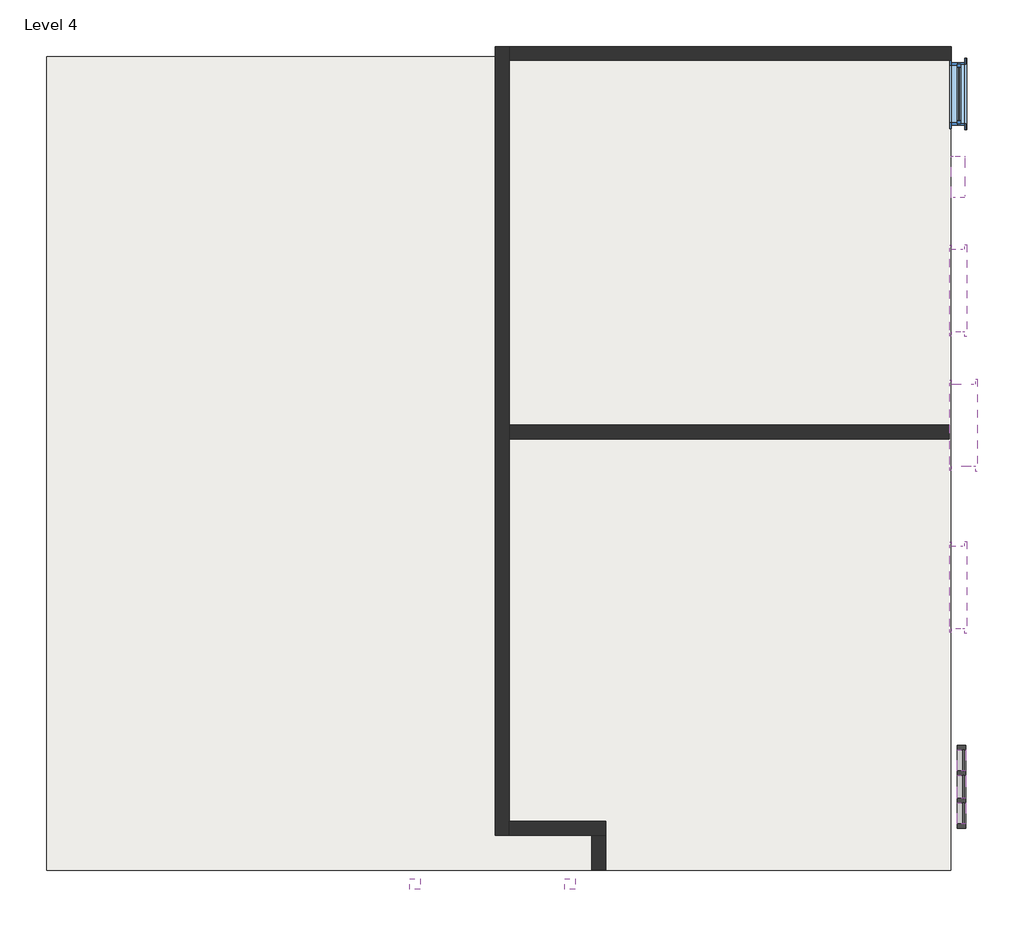
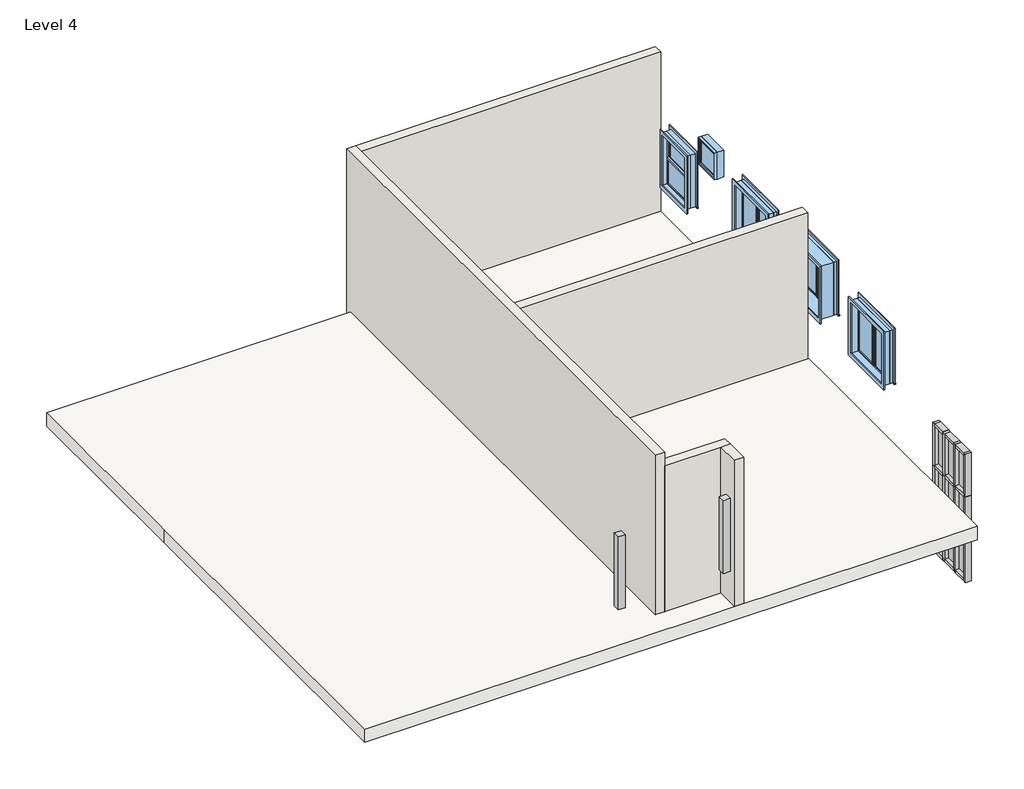
# One storey: 24 members, 9 plates, 5 walls, 5 windows, 2 proxies, 1 roof.
"""IFC4 building model written with IfcOpenShell, lengths in millimetres."""

from ifc_helpers import new_model, si_unit, frame, origin, place, context, project, spatial, polyline, outline, extrude, faceted_brep, transform, mapped, element, save
from components import member_ff1b7d8f, member_5ad95953, member_5aeb4b7d, member_9850ab14, member_fc2bd130, member_09852e99, system_panel_glazed_48942baa, system_panel_glazed_b83167b9, system_panel_glazed_fcfd29d5, system_panel_glazed_c81023b1, window_0862ab64, window_6544a982, window_31198920, window_6846e476

model = new_model("IFC4")

# Units and contexts
model_context = context("Model", 3, world=origin())
ifc_project = project(units=[si_unit("LENGTHUNIT", "METRE", prefix="MILLI")], contexts=[model_context])

# Site, building, storey
site = spatial("IfcSite", under=ifc_project)
building = spatial("IfcBuilding", under=site)
storey = spatial("IfcBuildingStorey", under=building, Name="Level 4", Elevation=10972.8)

# Proxies
placement = place(None, origin())
element("IfcBuildingElementProxy", 1, Name="Cornice", ObjectType="Cornice", at=placement, inside=storey, context=model_context, shape_type="SweptSolid", body=[
    extrude(outline(polyline([(-6354.4547188, -909.5189974), (-6354.4547188, -1061.9189974), (-6506.8547188, -1061.9189974), (-6506.8547188, -909.5189974), (-6354.4547188, -909.5189974)])), frame((0.0, 0.0, 12313.3022407), z_axis=(0.0, 0.0, 1.0), x_axis=(1.0, 0.0, 0.0)), (0.0, 0.0, 1.0), 1676.4),
])
element("IfcBuildingElementProxy", 2, Name="Cornice", ObjectType="Cornice", at=placement, inside=storey, context=model_context, shape_type="SweptSolid", body=[
    extrude(outline(polyline([(-4073.2084212, -909.5189974), (-4073.2084212, -1061.9189974), (-4225.6084212, -1061.9189974), (-4225.6084212, -909.5189974), (-4073.2084212, -909.5189974)])), frame((0.0, 0.0, 12347.4321664), z_axis=(0.0, 0.0, 1.0), x_axis=(1.0, 0.0, 0.0)), (0.0, 0.0, 1.0), 1676.4),
])

# Members
member_shape = member_ff1b7d8f(model_context)
element("IfcMember", 3, ObjectType="Rectangular Mullion : 2.5\" x 5\" rectangular", at=placement, inside=storey, context=model_context, shape_type="MappedRepresentation", body=[
    mapped(member_shape, transform((1611.5254876, 617.0832725, 9576.1019988), x_axis=(0.0, 0.0, -1.0), y_axis=(-1.0, 0.0, 0.0), z_axis=(0.0, 1.0, 0.0))),
])
member_2_shape = member_5ad95953(model_context)
element("IfcMember", 4, ObjectType="Rectangular Mullion : 2.5\" x 5\" rectangular", at=placement, inside=storey, context=model_context, shape_type="MappedRepresentation", body=[
    mapped(member_2_shape, transform((1611.5254876, 210.6832725, 9576.1019988), x_axis=(0.0, 0.0, -1.0), y_axis=(-1.0, 0.0, 0.0), z_axis=(0.0, 1.0, 0.0))),
])
element("IfcMember", 5, ObjectType="Rectangular Mullion : 2.5\" x 5\" rectangular", at=placement, inside=storey, context=model_context, shape_type="MappedRepresentation", body=[
    mapped(member_2_shape, transform((1611.5254876, 991.7332725, 9576.1019988), x_axis=(0.0, 0.0, -1.0), y_axis=(-1.0, 0.0, 0.0), z_axis=(0.0, 1.0, 0.0))),
])
member_3_shape = member_5aeb4b7d(model_context)
element("IfcMember", 6, ObjectType="Rectangular Mullion : 2.5\" x 5\" rectangular", at=placement, inside=storey, context=model_context, shape_type="MappedRepresentation", body=[
    mapped(member_3_shape, transform((1611.5254876, 274.1832725, 10558.2353321), x_axis=(0.0, 0.0, 1.0), y_axis=(-1.0, 0.0, 0.0), z_axis=(0.0, -1.0, 0.0))),
])
element("IfcMember", 7, ObjectType="Rectangular Mullion : 2.5\" x 5\" rectangular", at=placement, inside=storey, context=model_context, shape_type="MappedRepresentation", body=[
    mapped(member_3_shape, transform((1611.5254876, 274.1832725, 11540.3686655), x_axis=(0.0, 0.0, 1.0), y_axis=(-1.0, 0.0, 0.0), z_axis=(0.0, -1.0, 0.0))),
])
member_4_shape = member_9850ab14(model_context)
element("IfcMember", 8, ObjectType="Rectangular Mullion : 2.5\" x 5\" rectangular", at=placement, inside=storey, context=model_context, shape_type="MappedRepresentation", body=[
    mapped(member_4_shape, transform((1611.5254876, -100.4667275, 10558.2353321), x_axis=(0.0, 0.0, 1.0), y_axis=(-1.0, 0.0, 0.0), z_axis=(0.0, -1.0, 0.0))),
])
element("IfcMember", 9, ObjectType="Rectangular Mullion : 2.5\" x 5\" rectangular", at=placement, inside=storey, context=model_context, shape_type="MappedRepresentation", body=[
    mapped(member_4_shape, transform((1611.5254876, 680.5832725, 10558.2353321), x_axis=(0.0, 0.0, 1.0), y_axis=(-1.0, 0.0, 0.0), z_axis=(0.0, -1.0, 0.0))),
])
element("IfcMember", 10, ObjectType="Rectangular Mullion : 2.5\" x 5\" rectangular", at=placement, inside=storey, context=model_context, shape_type="MappedRepresentation", body=[
    mapped(member_4_shape, transform((1611.5254876, -100.4667275, 11540.3686655), x_axis=(0.0, 0.0, 1.0), y_axis=(-1.0, 0.0, 0.0), z_axis=(0.0, -1.0, 0.0))),
])
element("IfcMember", 11, ObjectType="Rectangular Mullion : 2.5\" x 5\" rectangular", at=placement, inside=storey, context=model_context, shape_type="MappedRepresentation", body=[
    mapped(member_4_shape, transform((1611.5254876, 680.5832725, 11540.3686655), x_axis=(0.0, 0.0, 1.0), y_axis=(-1.0, 0.0, 0.0), z_axis=(0.0, -1.0, 0.0))),
])
element("IfcMember", 12, ObjectType="Rectangular Mullion : 2.5\" x 5\" rectangular", at=placement, inside=storey, context=model_context, shape_type="MappedRepresentation", body=[
    mapped(member_2_shape, transform((1611.5254876, 680.5832725, 12522.5019988), x_axis=(0.0, 0.0, 1.0), y_axis=(-1.0, 0.0, 0.0), z_axis=(0.0, -1.0, 0.0))),
])
element("IfcMember", 13, ObjectType="Rectangular Mullion : 2.5\" x 5\" rectangular", at=placement, inside=storey, context=model_context, shape_type="MappedRepresentation", body=[
    mapped(member_2_shape, transform((1611.5254876, -100.4667275, 12522.5019988), x_axis=(0.0, 0.0, 1.0), y_axis=(-1.0, 0.0, 0.0), z_axis=(0.0, -1.0, 0.0))),
])
element("IfcMember", 14, ObjectType="Rectangular Mullion : 2.5\" x 5\" rectangular", at=placement, inside=storey, context=model_context, shape_type="MappedRepresentation", body=[
    mapped(member_shape, transform((1611.5254876, 274.1832725, 12522.5019988), x_axis=(0.0, 0.0, 1.0), y_axis=(-1.0, 0.0, 0.0), z_axis=(0.0, -1.0, 0.0))),
])
member_5_shape = member_fc2bd130(model_context)
element("IfcMember", 15, ObjectType="Rectangular Mullion : 2.5\" x 5\" rectangular", at=placement, inside=storey, context=model_context, shape_type="MappedRepresentation", body=[
    mapped(member_5_shape, transform((1611.5254876, 242.4332725, 9576.1019988), x_axis=(0.0, -1.0, 0.0), y_axis=(-1.0, 0.0, 0.0), z_axis=(0.0, 0.0, -1.0))),
])
element("IfcMember", 16, ObjectType="Rectangular Mullion : 2.5\" x 5\" rectangular", at=placement, inside=storey, context=model_context, shape_type="MappedRepresentation", body=[
    mapped(member_5_shape, transform((1611.5254876, 648.8332725, 9576.1019988), x_axis=(0.0, -1.0, 0.0), y_axis=(-1.0, 0.0, 0.0), z_axis=(0.0, 0.0, -1.0))),
])
element("IfcMember", 17, ObjectType="Rectangular Mullion : 2.5\" x 5\" rectangular", at=placement, inside=storey, context=model_context, shape_type="MappedRepresentation", body=[
    mapped(member_5_shape, transform((1611.5254876, 242.4332725, 10558.2353321), x_axis=(0.0, -1.0, 0.0), y_axis=(-1.0, 0.0, 0.0), z_axis=(0.0, 0.0, -1.0))),
])
element("IfcMember", 18, ObjectType="Rectangular Mullion : 2.5\" x 5\" rectangular", at=placement, inside=storey, context=model_context, shape_type="MappedRepresentation", body=[
    mapped(member_5_shape, transform((1611.5254876, 648.8332725, 10558.2353321), x_axis=(0.0, -1.0, 0.0), y_axis=(-1.0, 0.0, 0.0), z_axis=(0.0, 0.0, -1.0))),
])
element("IfcMember", 19, ObjectType="Rectangular Mullion : 2.5\" x 5\" rectangular", at=placement, inside=storey, context=model_context, shape_type="MappedRepresentation", body=[
    mapped(member_5_shape, transform((1611.5254876, 242.4332725, 11540.3686655), x_axis=(0.0, -1.0, 0.0), y_axis=(-1.0, 0.0, 0.0), z_axis=(0.0, 0.0, -1.0))),
])
element("IfcMember", 20, ObjectType="Rectangular Mullion : 2.5\" x 5\" rectangular", at=placement, inside=storey, context=model_context, shape_type="MappedRepresentation", body=[
    mapped(member_5_shape, transform((1611.5254876, 648.8332725, 11540.3686655), x_axis=(0.0, -1.0, 0.0), y_axis=(-1.0, 0.0, 0.0), z_axis=(0.0, 0.0, -1.0))),
])
member_6_shape = member_09852e99(model_context)
element("IfcMember", 21, ObjectType="Rectangular Mullion : 2.5\" x 5\" rectangular", at=placement, inside=storey, context=model_context, shape_type="MappedRepresentation", body=[
    mapped(member_6_shape, transform((1611.5254876, 1055.2332725, 11540.3686655), x_axis=(0.0, 1.0, 0.0), y_axis=(-1.0, 0.0, 0.0), z_axis=(0.0, 0.0, 1.0))),
])
element("IfcMember", 22, ObjectType="Rectangular Mullion : 2.5\" x 5\" rectangular", at=placement, inside=storey, context=model_context, shape_type="MappedRepresentation", body=[
    mapped(member_6_shape, transform((1611.5254876, 1055.2332725, 10558.2353321), x_axis=(0.0, 1.0, 0.0), y_axis=(-1.0, 0.0, 0.0), z_axis=(0.0, 0.0, 1.0))),
])
element("IfcMember", 23, ObjectType="Rectangular Mullion : 2.5\" x 5\" rectangular", at=placement, inside=storey, context=model_context, shape_type="MappedRepresentation", body=[
    mapped(member_6_shape, transform((1611.5254876, 1055.2332725, 12522.5019988), x_axis=(0.0, 1.0, 0.0), y_axis=(-1.0, 0.0, 0.0), z_axis=(0.0, 0.0, 1.0))),
])
element("IfcMember", 24, ObjectType="Rectangular Mullion : 2.5\" x 5\" rectangular", at=placement, inside=storey, context=model_context, shape_type="MappedRepresentation", body=[
    mapped(member_6_shape, transform((1611.5254876, -163.9667275, 11540.3686655), x_axis=(0.0, -1.0, 0.0), y_axis=(-1.0, 0.0, 0.0), z_axis=(0.0, 0.0, -1.0))),
])
element("IfcMember", 25, ObjectType="Rectangular Mullion : 2.5\" x 5\" rectangular", at=placement, inside=storey, context=model_context, shape_type="MappedRepresentation", body=[
    mapped(member_6_shape, transform((1611.5254876, -163.9667275, 10558.2353321), x_axis=(0.0, -1.0, 0.0), y_axis=(-1.0, 0.0, 0.0), z_axis=(0.0, 0.0, -1.0))),
])
element("IfcMember", 26, ObjectType="Rectangular Mullion : 2.5\" x 5\" rectangular", at=placement, inside=storey, context=model_context, shape_type="MappedRepresentation", body=[
    mapped(member_6_shape, transform((1611.5254876, -163.9667275, 9576.1019988), x_axis=(0.0, -1.0, 0.0), y_axis=(-1.0, 0.0, 0.0), z_axis=(0.0, 0.0, -1.0))),
])

# Plates
system_panel_glazed_shape = system_panel_glazed_48942baa(model_context)
element("IfcPlate", 27, ObjectType="System Panel : Glazed", at=placement, inside=storey, context=model_context, shape_type="MappedRepresentation", body=[
    mapped(system_panel_glazed_shape, transform((1611.5254876, 445.6332725, 9639.6019988), x_axis=(0.0, -1.0, 0.0), y_axis=(1.0, 0.0, 0.0), z_axis=(0.0, 0.0, 1.0))),
])
element("IfcPlate", 28, ObjectType="System Panel : Glazed", at=placement, inside=storey, context=model_context, shape_type="MappedRepresentation", body=[
    mapped(system_panel_glazed_shape, transform((1611.5254876, 445.6332725, 11572.1186655), x_axis=(0.0, -1.0, 0.0), y_axis=(1.0, 0.0, 0.0), z_axis=(0.0, 0.0, 1.0))),
])
system_panel_glazed_2_shape = system_panel_glazed_b83167b9(model_context)
element("IfcPlate", 29, ObjectType="System Panel : Glazed", at=placement, inside=storey, context=model_context, shape_type="MappedRepresentation", body=[
    mapped(system_panel_glazed_2_shape, transform((1611.5254876, 445.6332725, 10589.9853321), x_axis=(0.0, -1.0, 0.0), y_axis=(1.0, 0.0, 0.0), z_axis=(0.0, 0.0, 1.0))),
])
system_panel_glazed_3_shape = system_panel_glazed_fcfd29d5(model_context)
element("IfcPlate", 30, ObjectType="System Panel : Glazed", at=placement, inside=storey, context=model_context, shape_type="MappedRepresentation", body=[
    mapped(system_panel_glazed_3_shape, transform((1611.5254876, 836.1582725, 9639.6019988), x_axis=(0.0, -1.0, 0.0), y_axis=(1.0, 0.0, 0.0), z_axis=(0.0, 0.0, 1.0))),
])
element("IfcPlate", 31, ObjectType="System Panel : Glazed", at=placement, inside=storey, context=model_context, shape_type="MappedRepresentation", body=[
    mapped(system_panel_glazed_3_shape, transform((1611.5254876, 55.1082725, 9639.6019988), x_axis=(0.0, -1.0, 0.0), y_axis=(1.0, 0.0, 0.0), z_axis=(0.0, 0.0, 1.0))),
])
element("IfcPlate", 32, ObjectType="System Panel : Glazed", at=placement, inside=storey, context=model_context, shape_type="MappedRepresentation", body=[
    mapped(system_panel_glazed_3_shape, transform((1611.5254876, 836.1582725, 11572.1186655), x_axis=(0.0, -1.0, 0.0), y_axis=(1.0, 0.0, 0.0), z_axis=(0.0, 0.0, 1.0))),
])
element("IfcPlate", 33, ObjectType="System Panel : Glazed", at=placement, inside=storey, context=model_context, shape_type="MappedRepresentation", body=[
    mapped(system_panel_glazed_3_shape, transform((1611.5254876, 55.1082725, 11572.1186655), x_axis=(0.0, -1.0, 0.0), y_axis=(1.0, 0.0, 0.0), z_axis=(0.0, 0.0, 1.0))),
])
system_panel_glazed_4_shape = system_panel_glazed_c81023b1(model_context)
element("IfcPlate", 34, ObjectType="System Panel : Glazed", at=placement, inside=storey, context=model_context, shape_type="MappedRepresentation", body=[
    mapped(system_panel_glazed_4_shape, transform((1611.5254876, 836.1582725, 10589.9853321), x_axis=(0.0, -1.0, 0.0), y_axis=(1.0, 0.0, 0.0), z_axis=(0.0, 0.0, 1.0))),
])
element("IfcPlate", 35, ObjectType="System Panel : Glazed", at=placement, inside=storey, context=model_context, shape_type="MappedRepresentation", body=[
    mapped(system_panel_glazed_4_shape, transform((1611.5254876, 55.1082725, 10589.9853321), x_axis=(0.0, -1.0, 0.0), y_axis=(1.0, 0.0, 0.0), z_axis=(0.0, 0.0, 1.0))),
])

# Roof
element("IfcRoof", 36, ObjectType="Generic - 12\"", at=placement, inside=storey, context=model_context, shape_type="SweptSolid", body=[
    extrude(outline(polyline([(-11850.4745124, 11192.9609482), (1452.7754876, 11192.9609482), (1452.7754876, -783.1390518), (-11850.4745124, -783.1390518), (-11850.4745124, 6786.0609482), (-11850.4745124, 11192.9609482)])), frame((0.0, 0.0, 10972.8), z_axis=(0.0, 0.0, 1.0), x_axis=(1.0, 0.0, 0.0)), (0.0, 0.0, 1.0), 304.8),
])

# Walls
element("IfcWall", 37, ObjectType="Generic - 8\"", at=placement, inside=storey, context=model_context, shape_type="Brep", body=[
    faceted_brep([(-5246.4745124, 11345.3609482, 10972.8), (-5246.4745124, -265.5667275, 10972.8), (-5246.4745124, -265.5667275, 14935.2), (-5246.4745124, 11345.3609482, 14935.2), (-5043.2745124, 11345.3609482, 10972.8), (-5043.2745124, 11345.3609482, 14935.2), (-5043.2745124, 11142.1609482, 14935.2), (-5043.2745124, -265.5667275, 14935.2), (-5043.2745124, -265.5667275, 14630.4), (-5043.2745124, -265.5667275, 10972.8), (-5043.2745124, -62.3667275, 10972.8), (-5043.2745124, 5566.8609482, 10972.8), (-5043.2745124, 5770.0609482, 10972.8), (-5043.2745124, 11142.1609482, 10972.8)], [[[0, 1, 2, 3]], [[4, 5, 6, 7, 8, 9, 10, 11, 12, 13]], [[1, 0, 4, 13, 12, 11, 10, 9]], [[3, 2, 7, 6, 5]], [[0, 3, 5, 4]], [[2, 1, 9, 8, 7]]]),
])
element("IfcWall", 38, ObjectType="Generic - 8\"", at=placement, inside=storey, context=model_context, shape_type="Brep", body=[
    faceted_brep([(-5043.2745124, 11142.1609482, 10972.8), (1459.1254876, 11142.1609482, 10972.8), (1459.1254876, 11142.1609482, 14935.2), (-5043.2745124, 11142.1609482, 14935.2), (-5043.2745124, 11345.3609482, 10972.8), (-5043.2745124, 11345.3609482, 14935.2), (1459.1254876, 11345.3609482, 14935.2), (1459.1254876, 11345.3609482, 11277.6), (1459.1254876, 11345.3609482, 10972.8)], [[[0, 1, 2, 3]], [[4, 5, 6, 7, 8]], [[1, 0, 4, 8]], [[3, 2, 6, 5]], [[1, 8, 7, 6, 2]], [[0, 3, 5, 4]]]),
])
element("IfcWall", 39, ObjectType="Generic - 8\"", at=placement, inside=storey, context=model_context, shape_type="SweptSolid", body=[
    extrude(outline(polyline([(1433.7254876, 5566.8609482), (-5043.2745124, 5566.8609482), (-5043.2745124, 5770.0609482), (1433.7254876, 5770.0609482), (1433.7254876, 5566.8609482)])), frame((0.0, 0.0, 10972.8), z_axis=(0.0, 0.0, 1.0), x_axis=(1.0, 0.0, 0.0)), (0.0, 0.0, 1.0), 3657.6),
])
element("IfcWall", 40, ObjectType="Generic - 8\"", at=placement, inside=storey, context=model_context, shape_type="Brep", body=[
    faceted_brep([(-5043.2745124, -265.5667275, 10972.8), (-3824.0745124, -265.5667275, 10972.8), (-3620.8745124, -265.5667275, 10972.8), (-3620.8745124, -265.5667275, 14630.4), (-3824.0745124, -265.5667275, 14630.4), (-5043.2745124, -265.5667275, 14630.4), (-5043.2745124, -62.3667275, 10972.8), (-5043.2745124, -62.3667275, 14630.4), (-3620.8745124, -62.3667275, 14630.4), (-3620.8745124, -62.3667275, 10972.8)], [[[0, 1, 2, 3, 4, 5]], [[6, 7, 8, 9]], [[2, 1, 0, 6, 9]], [[5, 4, 3, 8, 7]], [[0, 5, 7, 6]], [[3, 2, 9, 8]]]),
])
element("IfcWall", 41, ObjectType="Generic - 8\"", at=placement, inside=storey, context=model_context, shape_type="SweptSolid", body=[
    extrude(outline(polyline([(-3824.0745124, -773.5667275), (-3824.0745124, -265.5667275), (-3620.8745124, -265.5667275), (-3620.8745124, -773.5667275), (-3824.0745124, -773.5667275)])), frame((0.0, 0.0, 10972.8), z_axis=(0.0, 0.0, 1.0), x_axis=(1.0, 0.0, 0.0)), (0.0, 0.0, 1.0), 3657.6),
])

# Windows
window_shape = window_0862ab64(model_context)
element("IfcWindow", 42, ObjectType="Casement Dbl with Trim : 48\" x 48\"", at=placement, inside=storey, context=model_context, shape_type="MappedRepresentation", body=[
    mapped(window_shape, transform((1541.6754876, 3382.4609482, 11430.0), x_axis=(0.0, -1.0, 0.0), y_axis=(1.0, 0.0, 0.0), z_axis=(0.0, 0.0, 1.0))),
])
element("IfcWindow", 43, ObjectType="Casement Dbl with Trim : 48\" x 48\"", at=placement, inside=storey, context=model_context, shape_type="MappedRepresentation", body=[
    mapped(window_shape, transform((1541.6754876, 7751.2609482, 11488.8204192), x_axis=(0.0, -1.0, 0.0), y_axis=(1.0, 0.0, 0.0), z_axis=(0.0, 0.0, 1.0))),
])
window_2_shape = window_6544a982(model_context)
element("IfcWindow", 44, ObjectType="Casement Dbl with Trim : 48\" x 48\"", at=placement, inside=storey, context=model_context, shape_type="MappedRepresentation", body=[
    mapped(window_2_shape, transform((1621.8754882, 5769.300673, 11495.6872891), x_axis=(0.0, -1.0, 0.0), y_axis=(1.0, 0.0, 0.0), z_axis=(0.0, 0.0, 1.0))),
])
window_3_shape = window_31198920(model_context)
element("IfcWindow", 45, ObjectType="Double Hung with Trim : 36\" x 48\"", at=placement, inside=storey, context=model_context, shape_type="MappedRepresentation", body=[
    mapped(window_3_shape, transform((1560.7254876, 10646.8609482, 10972.8), x_axis=(0.0, -1.0, 0.0), y_axis=(1.0, 0.0, 0.0), z_axis=(0.0, 0.0, 1.0))),
])
window_4_shape = window_6846e476(model_context)
element("IfcWindow", 46, ObjectType="Fixed : 24\" x 24\"", at=placement, inside=storey, context=model_context, shape_type="MappedRepresentation", body=[
    mapped(window_4_shape, transform((1560.7254876, 9465.7609482, 12304.4684583), x_axis=(0.0, 1.0, 0.0), y_axis=(-1.0, 0.0, 0.0), z_axis=(0.0, 0.0, 1.0))),
])

save(model, "model.ifc")

# Revit data of these elements
# Type "Rectangular Mullion : 2.5\" x 5\" rectangular"
#   built-in parameter 1007304 = 0.416667 (stored number, unit not read)
#   built-in parameter 1007301 = 0.104167 (stored number, unit not read)
#   built-in parameter 1007300 = 0.104167 (stored number, unit not read)
# Type "System Panel : Glazed"
#   Construction Type Id = "GSP4R"
#   Analytic Construction = "1/8 in Pilkington single glazing"
#   Visual Light Transmittance = 0.9
#   Solar Heat Gain Coefficient = 0.86
#   Heat Transfer Coefficient (U) = 1.18115 BTU/(h·ft²·°F)
# Type "Generic - 12\""
#   Assembly Code = "B1020"
#   Layers, outside or top first: 1' - 0" no material (function 1)
# Type "Generic - 8\""
#   Assembly Code = "B2010"
#   Layers, outside or top first: 0' - 8" no material (function 1)
# Type "Casement Dbl with Trim : 48\" x 48\""
#   Type Mark = "13"
#   Construction Type Id = "GSP4R"
#   Assembly Code = "B2020100"
#   Analytic Construction = "1/8 in Pilkington single glazing"
#   Visual Light Transmittance = 0.9
#   Solar Heat Gain Coefficient = 0.78
#   Heat Transfer Coefficient (U) = 0.6496 BTU/(h·ft²·°F)
#   Height = 4' - 0"
#   Default Sill Height = 3' - 0"
#   Trim Projection - Ext. = 0' - 0 1/2"
#   Trim Projection - Int. = 0' - 0 3/4"
#   Trim Width - Exterior = 0' - 3 1/2"
#   Trim Width - Interior = 0' - 3 1/2"
#   Width = 4' - 0"
#   Window Inset = 0' - 0 3/4"
#   Define Thermal Properties by = 1
#   Glass Pane Material = Glass
#   Sash Material = Sash
#   Trim Exterior Material = Trim
#   Trim Interior Material = Trim
#   Wall Closure = (empty or 0)
# Type "Double Hung with Trim : 36\" x 48\""
#   Type Mark = "16"
#   Construction Type Id = "GSP4R"
#   Assembly Code = "B2020100"
#   Analytic Construction = "1/8 in Pilkington single glazing"
#   Visual Light Transmittance = 0.9
#   Solar Heat Gain Coefficient = 0.78
#   Heat Transfer Coefficient (U) = 0.6496 BTU/(h·ft²·°F)
#   Height = 4' - 0"
#   Default Sill Height = 3' - 0"
#   Trim Projection - Ext. = 0' - 0 1/2"
#   Trim Projection - Int. = 0' - 0 3/4"
#   Trim Width - Exterior = 0' - 3 1/2"
#   Trim Width - Interior = 0' - 3 1/2"
#   Width = 3' - 0"
#   Window Inset = 0' - 0 3/4"
#   Define Thermal Properties by = 1
#   Glass Pane Material = Glass
#   Sash Material = Sash
#   Trim Exterior Material = Trim
#   Trim Interior Material = Trim
#   Wall Closure = (empty or 0)
# Type "Fixed : 24\" x 24\""
#   Type Mark = "3"
#   Construction Type Id = "GSP4R"
#   Assembly Code = "B2020100"
#   Analytic Construction = "1/8 in Pilkington single glazing"
#   Visual Light Transmittance = 0.9
#   Solar Heat Gain Coefficient = 0.78
#   Heat Transfer Coefficient (U) = 0.6496 BTU/(h·ft²·°F)
#   Height = 2' - 0"
#   Default Sill Height = 3' - 0"
#   Width = 2' - 0"
#   Window Inset = 0' - 0 3/4"
#   Define Thermal Properties by = 1
#   Glass Pane Material = Glass
#   Sash Material = Sash
#   Wall Closure = (empty or 0)
# Elements 1, 2 (IfcBuildingElementProxy, "Cornice")
#   Phase Created = New Construction
#   Materials on its faces: "Default Wall"
# Elements 3, 4, 5, 6, 7, 8, 9, 10, 11, 12, 13, 14, 15, 16, 17, 18, 19, 20, 21, 22, 23, 24, 25, 26 (IfcMember, "Rectangular Mullion : 2.5\" x 5\" rectangular")
#   Phase Created = New Construction
#   Materials on its faces: "Aluminum"
# Elements 27, 28, 29, 30, 31, 32, 33, 34, 35 (IfcPlate, "System Panel : Glazed")
#   Phase Created = New Construction
#   Materials on its faces: "Glass"
# Element 36 (IfcRoof, "Generic - 12\"")
#   built-in parameter 1001705 = 37 (stored number, unit not read)
#   built-in parameter 1001710 = 33615
#   Phase Created = New Construction
#   Materials on its faces: "Default Roof"
# Elements 37, 38 (IfcWall, "Generic - 8\"")
#   Top Offset = 0' - 0"
#   Base Offset = 0' - 0"
#   Unconnected Height = 13' - 0"
#   wall height = 13' - 0"
#   Phase Created = New Construction
#   Base Constraint = Level 4
#   Materials on its faces: "Default Wall"
# Elements 39, 40, 41 (IfcWall, "Generic - 8\"")
#   Top Offset = 0' - 0"
#   Base Offset = 0' - 0"
#   Unconnected Height = 12' - 0"
#   wall height = 12' - 0"
#   Phase Created = New Construction
#   Base Constraint = Level 4
#   Materials on its faces: "Default Wall"
# Element 42 (IfcWindow, "Casement Dbl with Trim : 48\" x 48\"")
#   Mark = "5"
#   Phase Created = New Construction
#   Materials on its faces: "Sash", "Trim", "Glass"
# Element 43 (IfcWindow, "Casement Dbl with Trim : 48\" x 48\"")
#   Mark = "7"
#   Phase Created = New Construction
#   Materials on its faces: "Sash", "Trim", "Glass"
# Element 44 (IfcWindow, "Casement Dbl with Trim : 48\" x 48\"")
#   Mark = "6"
#   Phase Created = New Construction
#   Materials on its faces: "Sash", "Trim", "Glass"
# Element 45 (IfcWindow, "Double Hung with Trim : 36\" x 48\"")
#   Mark = "8"
#   Phase Created = New Construction
#   Materials on its faces: "Sash", "Trim", "Glass"
# Element 46 (IfcWindow, "Fixed : 24\" x 24\"")
#   Mark = "3"
#   Phase Created = New Construction
#   Materials on its faces: "Sash", "Glass"
# Materials
#   "Glass": class "Glass", colour RGB 0 128 192, transparency 0.75, Description = "Soda Lime Glass", Cost = 0
#   "Sash": class "Wood", colour RGB 224 178 126, transparency 0
#   "Trim": class "Wood", colour RGB 224 178 126, transparency 0
#   "Default Wall": colour RGB 128 128 128, transparency 0
#   "Aluminum": class "Metal", colour RGB 247 247 247, transparency 0, Description = "Aluminum 6061", Cost = 0
#   "Default Roof": colour RGB 88 101 114, transparency 0
